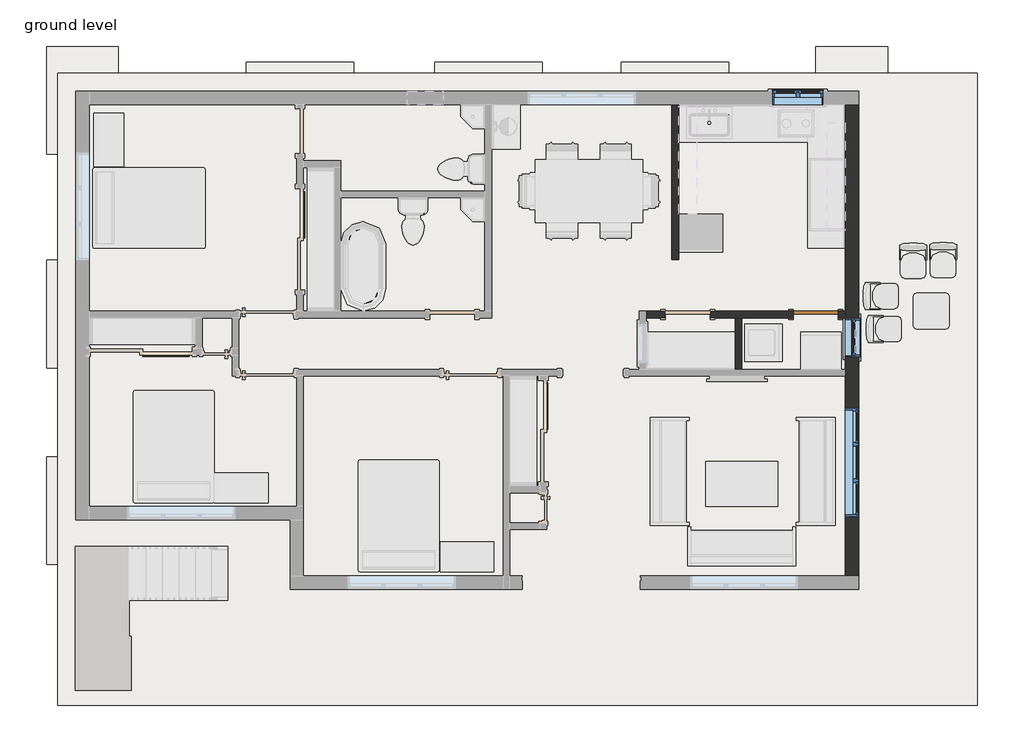
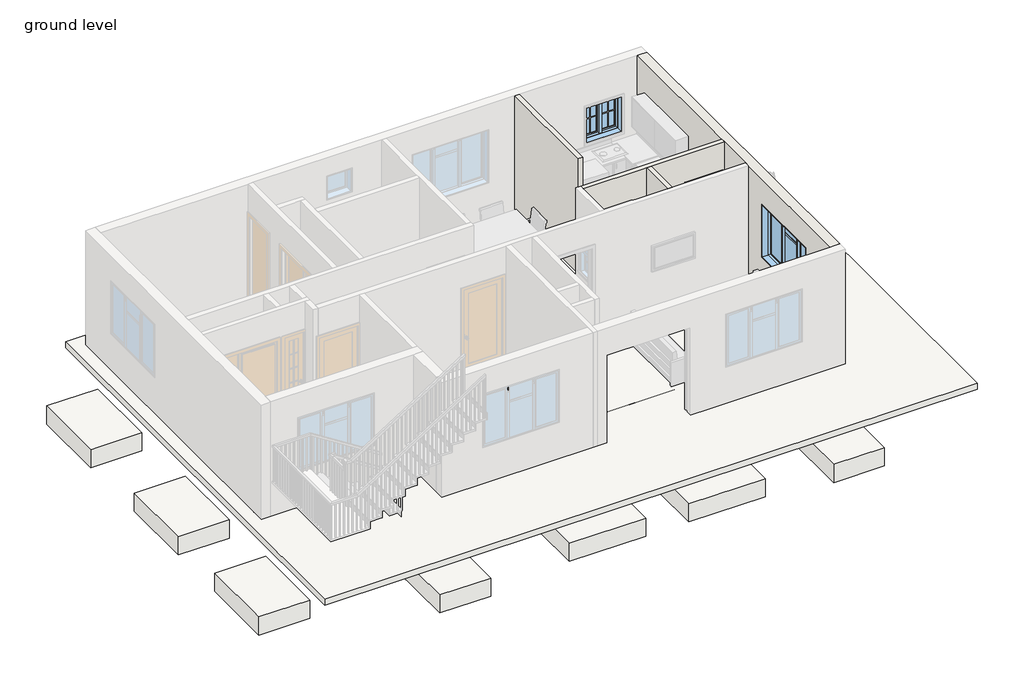
# One storey, part 2 of 4: 18 beams, 15 slabs, 4 walls, 3 windows, 1 door.
"""IFC4 building model written with IfcOpenShell, lengths in millimetres."""

from ifc_helpers import new_model, si_unit, frame, origin, place, context, project, spatial, polyline, outline, extrude, faceted_brep, transform, mapped, element, save
from components import door_214872d5, window_339605e1, window_7a1f68bc, window_251dd907

model = new_model("IFC4")

# Units and contexts
model_context = context("Model", 3, world=origin())
ifc_project = project(units=[si_unit("LENGTHUNIT", "METRE", prefix="MILLI")], contexts=[model_context])

# Site, building, storey
site = spatial("IfcSite", under=ifc_project)
building = spatial("IfcBuilding", under=site)
storey = spatial("IfcBuildingStorey", under=building, Name="ground level", Elevation=609.6)

# Beams
placement = place(None, origin())
element("IfcBeam", 1, ObjectType="Concrete-Rectangular Beam", at=placement, inside=storey, context=model_context, shape_type="Brep", body=[
    faceted_brep([(-8931.9263529, 6644.5661978, 609.6), (-8931.9263529, 6415.9661978, 609.6), (-5521.9763529, 6415.9661978, 609.6), (-5293.3763529, 6415.9661978, 609.6), (-2264.4263529, 6415.9661978, 609.6), (-2035.8263529, 6415.9661978, 609.6), (897.8736471, 6415.9661978, 609.6), (1126.4736471, 6415.9661978, 609.6), (3901.4236471, 6415.9661978, 609.6), (3901.4236471, 6644.5661978, 609.6), (1164.5736471, 6644.5661978, 609.6), (1164.5736471, 6454.0661978, 609.6), (859.7736471, 6454.0661978, 609.6), (859.7736471, 6644.5661978, 609.6), (-1997.7263529, 6644.5661978, 609.6), (-1997.7263529, 6454.0661978, 609.6), (-2302.5263529, 6454.0661978, 609.6), (-2302.5263529, 6644.5661978, 609.6), (-5198.1263529, 6644.5661978, 609.6), (-5198.1263529, 6454.0661978, 609.6), (-5502.9263529, 6454.0661978, 609.6), (-5502.9263529, 6644.5661978, 609.6), (-8931.9263529, 6415.9661978, 304.8), (-5521.9763529, 6415.9661978, 304.8), (-5293.3763529, 6415.9661978, 304.8), (-2264.4263529, 6415.9661978, 304.8), (-2035.8263529, 6415.9661978, 304.8), (897.8736471, 6415.9661978, 304.8), (1126.4736471, 6415.9661978, 304.8), (3901.4236471, 6415.9661978, 304.8), (-8931.9263529, 6644.5661978, 304.8), (-5502.9263529, 6644.5661978, 304.8), (-5502.9263529, 6454.0661978, 304.8), (-5198.1263529, 6454.0661978, 304.8), (-5198.1263529, 6644.5661978, 304.8), (-2302.5263529, 6644.5661978, 304.8), (-2302.5263529, 6454.0661978, 304.8), (-1997.7263529, 6454.0661978, 304.8), (-1997.7263529, 6644.5661978, 304.8), (859.7736471, 6644.5661978, 304.8), (859.7736471, 6454.0661978, 304.8), (1164.5736471, 6454.0661978, 304.8), (1164.5736471, 6644.5661978, 304.8), (3901.4236471, 6644.5661978, 304.8)], [[[0, 1, 2, 3, 4, 5, 6, 7, 8, 9, 10, 11, 12, 13, 14, 15, 16, 17, 18, 19, 20, 21]], [[1, 22, 23, 24, 25, 26, 27, 28, 29, 8, 7, 6, 5, 4, 3, 2]], [[22, 30, 31, 32, 33, 34, 35, 36, 37, 38, 39, 40, 41, 42, 43, 29, 28, 27, 26, 25, 24, 23]], [[42, 10, 9, 43]], [[1, 0, 30, 22]], [[33, 19, 18, 34]], [[19, 33, 32, 20]], [[20, 32, 31, 21]], [[37, 15, 14, 38]], [[15, 37, 36, 16]], [[16, 36, 35, 17]], [[41, 11, 10, 42]], [[11, 41, 40, 12]], [[12, 40, 39, 13]], [[9, 8, 29, 43]], [[30, 0, 21, 31]], [[34, 18, 17, 35]], [[38, 14, 13, 39]]]),
])
element("IfcBeam", 2, ObjectType="Concrete-Rectangular Beam", at=placement, inside=storey, context=model_context, shape_type="Brep", body=[
    faceted_brep([(4130.0236471, 1748.7161978, 609.6), (3901.4236471, 1748.7161978, 609.6), (3901.4236471, 1729.6661978, 609.6), (3901.4236471, 34.2161978, 609.6), (3901.4236471, -194.3838022, 609.6), (3901.4236471, -588.0838022, 609.6), (3901.4236471, -816.6838022, 609.6), (3901.4236471, -1470.7338022, 609.6), (4130.0236471, -1470.7338022, 609.6), (3901.4236471, 1748.7161978, 304.8), (3901.4236471, 1729.6661978, 304.8), (3901.4236471, 34.2161978, 304.8), (3901.4236471, -194.3838022, 304.8), (3901.4236471, -588.0838022, 304.8), (3901.4236471, -816.6838022, 304.8), (3901.4236471, -1470.7338022, 304.8), (4130.0236471, 1748.7161978, 304.8), (4130.0236471, -1470.7338022, 304.8)], [[[0, 1, 2, 3, 4, 5, 6, 7, 8]], [[1, 9, 10, 11, 12, 13, 14, 15, 7, 6, 5, 4, 3, 2]], [[9, 16, 17, 15, 14, 13, 12, 11, 10]], [[16, 0, 8, 17]], [[1, 0, 16, 9]], [[8, 7, 15, 17]]]),
    faceted_brep([(3901.4236471, 6377.8661978, 609.6), (4130.0236471, 6377.8661978, 609.6), (4130.0236471, 6377.8661978, 304.8), (3901.4236471, 6377.8661978, 304.8), (4130.0236471, 2053.5161978, 609.6), (3901.4236471, 2053.5161978, 609.6), (3901.4236471, 2053.5161978, 304.8), (4130.0236471, 2053.5161978, 304.8), (3901.4236471, 5558.7161978, 609.6), (3901.4236471, 5330.1161978, 609.6), (3901.4236471, 5044.3661978, 609.6), (3901.4236471, 4815.7661978, 609.6), (3901.4236471, 3012.3661978, 609.6), (3901.4236471, 2783.7661978, 609.6), (3901.4236471, 5558.7161978, 304.8), (3901.4236471, 5330.1161978, 304.8), (3901.4236471, 5044.3661978, 304.8), (3901.4236471, 4815.7661978, 304.8), (3901.4236471, 3012.3661978, 304.8), (3901.4236471, 2783.7661978, 304.8)], [[[0, 1, 2, 3]], [[4, 5, 6, 7]], [[1, 0, 8, 9, 10, 11, 12, 13, 5, 4]], [[0, 3, 14, 15, 16, 17, 18, 19, 6, 5, 13, 12, 11, 10, 9, 8]], [[3, 2, 7, 6, 19, 18, 17, 16, 15, 14]], [[2, 1, 4, 7]]]),
])
element("IfcBeam", 3, ObjectType="Concrete-Rectangular Beam", at=placement, inside=storey, context=model_context, shape_type="Brep", body=[
    faceted_brep([(3901.4236471, -1737.4338022, 609.6), (3901.4236471, -1508.8338022, 609.6), (-1731.0263529, -1508.8338022, 609.6), (-1959.6263529, -1508.8338022, 609.6), (-5293.3763529, -1508.8338022, 609.6), (-5293.3763529, -1737.4338022, 609.6), (-1997.7263529, -1737.4338022, 609.6), (-1997.7263529, -1546.9338022, 609.6), (-1692.9263529, -1546.9338022, 609.6), (-1692.9263529, -1737.4338022, 609.6), (859.7736471, -1737.4338022, 609.6), (859.7736471, -1546.9338022, 609.6), (1164.5736471, -1546.9338022, 609.6), (1164.5736471, -1737.4338022, 609.6), (3901.4236471, -1508.8338022, 304.8), (-1731.0263529, -1508.8338022, 304.8), (-1959.6263529, -1508.8338022, 304.8), (-5293.3763529, -1508.8338022, 304.8), (3901.4236471, -1737.4338022, 304.8), (1164.5736471, -1737.4338022, 304.8), (1164.5736471, -1546.9338022, 304.8), (859.7736471, -1546.9338022, 304.8), (859.7736471, -1737.4338022, 304.8), (-1692.9263529, -1737.4338022, 304.8), (-1692.9263529, -1546.9338022, 304.8), (-1997.7263529, -1546.9338022, 304.8), (-1997.7263529, -1737.4338022, 304.8), (-5293.3763529, -1737.4338022, 304.8)], [[[0, 1, 2, 3, 4, 5, 6, 7, 8, 9, 10, 11, 12, 13]], [[1, 14, 15, 16, 17, 4, 3, 2]], [[14, 18, 19, 20, 21, 22, 23, 24, 25, 26, 27, 17, 16, 15]], [[26, 6, 5, 27]], [[1, 0, 18, 14]], [[21, 11, 10, 22]], [[11, 21, 20, 12]], [[12, 20, 19, 13]], [[25, 7, 6, 26]], [[7, 25, 24, 8]], [[8, 24, 23, 9]], [[5, 4, 17, 27]], [[18, 0, 13, 19]], [[22, 10, 9, 23]]]),
])
element("IfcBeam", 4, ObjectType="Concrete-Rectangular Beam", at=placement, inside=storey, context=model_context, shape_type="Brep", body=[
    faceted_brep([(-5293.3763529, 6415.9661978, 609.6), (-5521.9763529, 6415.9661978, 609.6), (-5521.9763529, 3012.3661978, 609.6), (-5521.9763529, 2783.7661978, 609.6), (-5521.9763529, 1958.2661978, 609.6), (-5521.9763529, 1729.6661978, 609.6), (-5521.9763529, -327.7338022, 609.6), (-5521.9763529, -556.3338022, 609.6), (-5521.9763529, -1470.7338022, 609.6), (-5293.3763529, -1470.7338022, 609.6), (-5293.3763529, 1729.6661978, 609.6), (-5401.3263529, 1729.6661978, 609.6), (-5401.3263529, 1958.2661978, 609.6), (-5293.3763529, 1958.2661978, 609.6), (-5293.3763529, 2783.7661978, 609.6), (-5293.3763529, 3012.3661978, 609.6), (-5293.3763529, 5330.1161978, 609.6), (-5293.3763529, 5558.7161978, 609.6), (-5293.3763529, 6415.9661978, 304.8), (-5293.3763529, 1958.2661978, 304.8), (-5293.3763529, 2783.7661978, 304.8), (-5293.3763529, 3012.3661978, 304.8), (-5293.3763529, 5330.1161978, 304.8), (-5293.3763529, 5558.7161978, 304.8), (-5521.9763529, 6415.9661978, 304.8), (-5401.3263529, 1958.2661978, 304.8), (-5401.3263529, 1729.6661978, 304.8), (-5293.3763529, 1729.6661978, 304.8), (-5293.3763529, -1470.7338022, 304.8), (-5521.9763529, -1470.7338022, 304.8), (-5521.9763529, -556.3338022, 304.8), (-5521.9763529, -327.7338022, 304.8), (-5521.9763529, 1729.6661978, 304.8), (-5521.9763529, 1958.2661978, 304.8), (-5521.9763529, 2783.7661978, 304.8), (-5521.9763529, 3012.3661978, 304.8)], [[[0, 1, 2, 3, 4, 5, 6, 7, 8, 9, 10, 11, 12, 13, 14, 15, 16, 17]], [[18, 0, 17, 16, 15, 14, 13, 19, 20, 21, 22, 23]], [[24, 18, 23, 22, 21, 20, 19, 25, 26, 27, 28, 29, 30, 31, 32, 33, 34, 35]], [[1, 24, 35, 34, 33, 32, 31, 30, 29, 8, 7, 6, 5, 4, 3, 2]], [[1, 0, 18, 24]], [[9, 8, 29, 28]], [[12, 25, 19, 13]], [[26, 11, 10, 27]], [[11, 26, 25, 12]], [[9, 28, 27, 10]]]),
])
element("IfcBeam", 5, ObjectType="Concrete-Rectangular Beam", at=placement, inside=storey, context=model_context, shape_type="SweptSolid", body=[
    extrude(outline(polyline([(-5521.9763529, -327.7338022), (-5521.9763529, -556.3338022), (-8931.9263529, -556.3338022), (-8931.9263529, -327.7338022), (-5521.9763529, -327.7338022)])), frame((0.0, 0.0, 304.8), z_axis=(0.0, 0.0, 1.0), x_axis=(1.0, 0.0, 0.0)), (0.0, 0.0, 1.0), 304.8),
])
element("IfcBeam", 6, ObjectType="Concrete-Rectangular Beam", at=placement, inside=storey, context=model_context, shape_type="Brep", body=[
    faceted_brep([(-9160.5263529, 6720.7661978, 609.6), (-8931.9263529, 6720.7661978, 609.6), (-8931.9263529, 6720.7661978, 304.8), (-9160.5263529, 6720.7661978, 304.8), (-9160.5263529, 6682.6661978, 609.6), (-8931.9263529, 6682.6661978, 609.6), (-8931.9263529, 6682.6661978, 304.8), (-9160.5263529, 6682.6661978, 304.8)], [[[0, 1, 2, 3]], [[1, 0, 4, 5]], [[2, 1, 5, 6]], [[3, 2, 6, 7]], [[0, 3, 7, 4]], [[5, 4, 7, 6]]]),
    faceted_brep([(-9160.5263529, 6377.8661978, 609.6), (-8931.9263529, 6377.8661978, 609.6), (-8931.9263529, 6377.8661978, 304.8), (-9160.5263529, 6377.8661978, 304.8), (-8931.9263529, 3050.4661978, 609.6), (-9160.5263529, 3050.4661978, 609.6), (-9160.5263529, 3050.4661978, 304.8), (-8931.9263529, 3050.4661978, 304.8)], [[[0, 1, 2, 3]], [[4, 5, 6, 7]], [[1, 0, 5, 4]], [[2, 1, 4, 7]], [[3, 2, 7, 6]], [[0, 3, 6, 5]]]),
    faceted_brep([(-8931.9263529, -289.6338022, 609.6), (-9160.5263529, -289.6338022, 609.6), (-9160.5263529, -289.6338022, 304.8), (-8931.9263529, -289.6338022, 304.8), (-9160.5263529, 2745.6661978, 609.6), (-8931.9263529, 2745.6661978, 609.6), (-8931.9263529, 2745.6661978, 304.8), (-9160.5263529, 2745.6661978, 304.8), (-8931.9263529, 1729.6661978, 609.6), (-8931.9263529, 1958.2661978, 609.6), (-8931.9263529, 1729.6661978, 304.8), (-8931.9263529, 1958.2661978, 304.8)], [[[0, 1, 2, 3]], [[4, 5, 6, 7]], [[1, 0, 8, 9, 5, 4]], [[0, 3, 10, 11, 6, 5, 9, 8]], [[3, 2, 7, 6, 11, 10]], [[2, 1, 4, 7]]]),
])
element("IfcBeam", 7, ObjectType="Concrete-Rectangular Beam", at=placement, inside=storey, context=model_context, shape_type="Brep", body=[
    faceted_brep([(-8931.9263529, 3012.3661978, 609.6), (-8931.9263529, 2783.7661978, 609.6), (-5521.9763529, 2783.7661978, 609.6), (-5521.9763529, 3012.3661978, 609.6), (-8931.9263529, 2783.7661978, 304.8), (-5521.9763529, 2783.7661978, 304.8), (-8931.9263529, 3012.3661978, 304.8), (-5521.9763529, 3012.3661978, 304.8)], [[[0, 1, 2, 3]], [[1, 4, 5, 2]], [[4, 6, 7, 5]], [[6, 0, 3, 7]], [[1, 0, 6, 4]], [[3, 2, 5, 7]]]),
    faceted_brep([(3901.4236471, 3012.3661978, 609.6), (3901.4236471, 2783.7661978, 609.6), (3901.4236471, 2783.7661978, 304.8), (3901.4236471, 3012.3661978, 304.8), (-5293.3763529, 2783.7661978, 609.6), (-5293.3763529, 3012.3661978, 609.6), (-5293.3763529, 3012.3661978, 304.8), (-5293.3763529, 2783.7661978, 304.8), (1126.4736471, 3012.3661978, 609.6), (897.8736471, 3012.3661978, 609.6), (-2035.8263529, 3012.3661978, 609.6), (-2264.4263529, 3012.3661978, 609.6), (-4601.2263529, 3012.3661978, 609.6), (-4829.8263529, 3012.3661978, 609.6), (351.7736471, 2783.7661978, 609.6), (580.3736471, 2783.7661978, 609.6), (1977.3736471, 2783.7661978, 609.6), (2205.9736471, 2783.7661978, 609.6), (351.7736471, 2783.7661978, 304.8), (580.3736471, 2783.7661978, 304.8), (1977.3736471, 2783.7661978, 304.8), (2205.9736471, 2783.7661978, 304.8), (-4829.8263529, 3012.3661978, 304.8), (-4601.2263529, 3012.3661978, 304.8), (-2264.4263529, 3012.3661978, 304.8), (-2035.8263529, 3012.3661978, 304.8), (897.8736471, 3012.3661978, 304.8), (1126.4736471, 3012.3661978, 304.8)], [[[0, 1, 2, 3]], [[4, 5, 6, 7]], [[1, 0, 8, 9, 10, 11, 12, 13, 5, 4, 14, 15, 16, 17]], [[2, 1, 17, 16, 15, 14, 4, 7, 18, 19, 20, 21]], [[3, 2, 21, 20, 19, 18, 7, 6, 22, 23, 24, 25, 26, 27]], [[0, 3, 27, 26, 25, 24, 23, 22, 6, 5, 13, 12, 11, 10, 9, 8]]]),
])
element("IfcBeam", 8, ObjectType="Concrete-Rectangular Beam", at=placement, inside=storey, context=model_context, shape_type="Brep", body=[
    faceted_brep([(-8931.9263529, 1958.2661978, 609.6), (-8931.9263529, 1729.6661978, 609.6), (-5521.9763529, 1729.6661978, 609.6), (-5521.9763529, 1958.2661978, 609.6), (-8931.9263529, 1729.6661978, 304.8), (-5521.9763529, 1729.6661978, 304.8), (-8931.9263529, 1958.2661978, 304.8), (-5521.9763529, 1958.2661978, 304.8)], [[[0, 1, 2, 3]], [[1, 4, 5, 2]], [[4, 6, 7, 5]], [[6, 0, 3, 7]], [[1, 0, 6, 4]], [[3, 2, 5, 7]]]),
    faceted_brep([(3901.4236471, 1958.2661978, 609.6), (3901.4236471, 1748.7161978, 609.6), (3901.4236471, 1729.6661978, 609.6), (3901.4236471, 1729.6661978, 304.8), (3901.4236471, 1748.7161978, 304.8), (3901.4236471, 1958.2661978, 304.8), (618.4736471, 1729.6661978, 609.6), (618.4736471, 1958.2661978, 609.6), (618.4736471, 1958.2661978, 304.8), (618.4736471, 1729.6661978, 304.8), (2205.9736471, 1958.2661978, 609.6), (1977.3736471, 1958.2661978, 609.6), (1977.3736471, 1958.2661978, 304.8), (2205.9736471, 1958.2661978, 304.8)], [[[0, 1, 2, 3, 4, 5]], [[6, 7, 8, 9]], [[2, 1, 0, 10, 11, 7, 6]], [[3, 2, 6, 9]], [[5, 4, 3, 9, 8, 12, 13]], [[0, 5, 13, 12, 8, 7, 11, 10]]]),
    faceted_brep([(-5096.5263529, 1729.6661978, 609.6), (-5096.5263529, 1958.2661978, 609.6), (-5096.5263529, 1958.2661978, 304.8), (-5096.5263529, 1729.6661978, 304.8), (313.6736471, 1958.2661978, 609.6), (313.6736471, 1729.6661978, 609.6), (313.6736471, 1729.6661978, 304.8), (313.6736471, 1958.2661978, 304.8), (-1959.6263529, 1729.6661978, 609.6), (-1731.0263529, 1729.6661978, 609.6), (-1959.6263529, 1729.6661978, 304.8), (-1731.0263529, 1729.6661978, 304.8)], [[[0, 1, 2, 3]], [[4, 5, 6, 7]], [[1, 0, 8, 9, 5, 4]], [[0, 3, 10, 11, 6, 5, 9, 8]], [[3, 2, 7, 6, 11, 10]], [[2, 1, 4, 7]]]),
])
element("IfcBeam", 9, ObjectType="Concrete-Rectangular Beam", at=placement, inside=storey, context=model_context, shape_type="Brep", body=[
    faceted_brep([(-1959.6263529, -1508.8338022, 609.6), (-1731.0263529, -1508.8338022, 609.6), (-1731.0263529, -816.6838022, 609.6), (-1731.0263529, -588.0838022, 609.6), (-1731.0263529, -194.3838022, 609.6), (-1731.0263529, 34.2161978, 609.6), (-1731.0263529, 1729.6661978, 609.6), (-1959.6263529, 1729.6661978, 609.6), (-1959.6263529, -1508.8338022, 304.8), (-1959.6263529, 1729.6661978, 304.8), (-1731.0263529, -1508.8338022, 304.8), (-1731.0263529, 1729.6661978, 304.8), (-1731.0263529, 34.2161978, 304.8), (-1731.0263529, -194.3838022, 304.8), (-1731.0263529, -588.0838022, 304.8), (-1731.0263529, -816.6838022, 304.8)], [[[0, 1, 2, 3, 4, 5, 6, 7]], [[8, 0, 7, 9]], [[10, 8, 9, 11, 12, 13, 14, 15]], [[1, 10, 15, 14, 13, 12, 11, 6, 5, 4, 3, 2]], [[1, 0, 8, 10]], [[7, 6, 11, 9]]]),
])
element("IfcBeam", 10, ObjectType="Concrete-Rectangular Beam", at=placement, inside=storey, context=model_context, shape_type="SweptSolid", body=[
    extrude(outline(polyline([(3901.4236471, -588.0838022), (3901.4236471, -816.6838022), (-1731.0263529, -816.6838022), (-1731.0263529, -588.0838022), (3901.4236471, -588.0838022)])), frame((0.0, 0.0, 304.8), z_axis=(0.0, 0.0, 1.0), x_axis=(1.0, 0.0, 0.0)), (0.0, 0.0, 1.0), 304.8),
])
element("IfcBeam", 11, ObjectType="Concrete-Rectangular Beam", at=placement, inside=storey, context=model_context, shape_type="SweptSolid", body=[
    extrude(outline(polyline([(3901.4236471, 34.2161978), (3901.4236471, -194.3838022), (-1731.0263529, -194.3838022), (-1731.0263529, 34.2161978), (3901.4236471, 34.2161978)])), frame((0.0, 0.0, 304.8), z_axis=(0.0, 0.0, 1.0), x_axis=(1.0, 0.0, 0.0)), (0.0, 0.0, 1.0), 304.8),
])
element("IfcBeam", 12, ObjectType="Concrete-Rectangular Beam", at=placement, inside=storey, context=model_context, shape_type="Brep", body=[
    faceted_brep([(3901.4236471, 5330.1161978, 609.6), (3901.4236471, 5558.7161978, 609.6), (1126.4736471, 5558.7161978, 609.6), (897.8736471, 5558.7161978, 609.6), (-2035.8263529, 5558.7161978, 609.6), (-2264.4263529, 5558.7161978, 609.6), (-5293.3763529, 5558.7161978, 609.6), (-5293.3763529, 5330.1161978, 609.6), (-4829.8263529, 5330.1161978, 609.6), (-4601.2263529, 5330.1161978, 609.6), (-2264.4263529, 5330.1161978, 609.6), (-2035.8263529, 5330.1161978, 609.6), (897.8736471, 5330.1161978, 609.6), (1126.4736471, 5330.1161978, 609.6), (3901.4236471, 5330.1161978, 304.8), (-5293.3763529, 5330.1161978, 304.8), (-4829.8263529, 5330.1161978, 304.8), (-4601.2263529, 5330.1161978, 304.8), (-2264.4263529, 5330.1161978, 304.8), (-2035.8263529, 5330.1161978, 304.8), (897.8736471, 5330.1161978, 304.8), (1126.4736471, 5330.1161978, 304.8), (3901.4236471, 5558.7161978, 304.8), (-5293.3763529, 5558.7161978, 304.8), (-2264.4263529, 5558.7161978, 304.8), (-2035.8263529, 5558.7161978, 304.8), (897.8736471, 5558.7161978, 304.8), (1126.4736471, 5558.7161978, 304.8)], [[[0, 1, 2, 3, 4, 5, 6, 7, 8, 9, 10, 11, 12, 13]], [[14, 0, 13, 12, 11, 10, 9, 8, 7, 15, 16, 17, 18, 19, 20, 21]], [[22, 14, 21, 20, 19, 18, 17, 16, 15, 23, 24, 25, 26, 27]], [[1, 22, 27, 26, 25, 24, 23, 6, 5, 4, 3, 2]], [[1, 0, 14, 22]], [[7, 6, 23, 15]]]),
])
element("IfcBeam", 13, ObjectType="Concrete-Rectangular Beam", at=placement, inside=storey, context=model_context, shape_type="Brep", body=[
    faceted_brep([(3901.4236471, 4815.7661978, 609.6), (3901.4236471, 5044.3661978, 609.6), (1126.4736471, 5044.3661978, 609.6), (897.8736471, 5044.3661978, 609.6), (-2035.8263529, 5044.3661978, 609.6), (-2264.4263529, 5044.3661978, 609.6), (-4601.2263529, 5044.3661978, 609.6), (-4601.2263529, 4815.7661978, 609.6), (-2264.4263529, 4815.7661978, 609.6), (-2035.8263529, 4815.7661978, 609.6), (897.8736471, 4815.7661978, 609.6), (1126.4736471, 4815.7661978, 609.6), (3901.4236471, 4815.7661978, 304.8), (-4601.2263529, 4815.7661978, 304.8), (-2264.4263529, 4815.7661978, 304.8), (-2035.8263529, 4815.7661978, 304.8), (897.8736471, 4815.7661978, 304.8), (1126.4736471, 4815.7661978, 304.8), (3901.4236471, 5044.3661978, 304.8), (-4601.2263529, 5044.3661978, 304.8), (-2264.4263529, 5044.3661978, 304.8), (-2035.8263529, 5044.3661978, 304.8), (897.8736471, 5044.3661978, 304.8), (1126.4736471, 5044.3661978, 304.8)], [[[0, 1, 2, 3, 4, 5, 6, 7, 8, 9, 10, 11]], [[12, 0, 11, 10, 9, 8, 7, 13, 14, 15, 16, 17]], [[18, 12, 17, 16, 15, 14, 13, 19, 20, 21, 22, 23]], [[1, 18, 23, 22, 21, 20, 19, 6, 5, 4, 3, 2]], [[1, 0, 12, 18]], [[7, 6, 19, 13]]]),
])
element("IfcBeam", 14, ObjectType="Concrete-Rectangular Beam", at=placement, inside=storey, context=model_context, shape_type="Brep", body=[
    faceted_brep([(-4829.8263529, 3012.3661978, 609.6), (-4601.2263529, 3012.3661978, 609.6), (-4601.2263529, 4815.7661978, 609.6), (-4601.2263529, 5044.3661978, 609.6), (-4601.2263529, 5330.1161978, 609.6), (-4829.8263529, 5330.1161978, 609.6), (-4829.8263529, 3012.3661978, 304.8), (-4829.8263529, 5330.1161978, 304.8), (-4601.2263529, 3012.3661978, 304.8), (-4601.2263529, 5330.1161978, 304.8), (-4601.2263529, 5044.3661978, 304.8), (-4601.2263529, 4815.7661978, 304.8)], [[[0, 1, 2, 3, 4, 5]], [[6, 0, 5, 7]], [[8, 6, 7, 9, 10, 11]], [[1, 8, 11, 10, 9, 4, 3, 2]], [[1, 0, 6, 8]], [[5, 4, 9, 7]]]),
])
element("IfcBeam", 15, ObjectType="Concrete-Rectangular Beam", at=placement, inside=storey, context=model_context, shape_type="SweptSolid", body=[
    extrude(outline(polyline([(-2035.8263529, 3012.3661978), (-2264.4263529, 3012.3661978), (-2264.4263529, 4815.7661978), (-2035.8263529, 4815.7661978), (-2035.8263529, 3012.3661978)])), frame((0.0, 0.0, 304.8), z_axis=(0.0, 0.0, 1.0), x_axis=(1.0, 0.0, 0.0)), (0.0, 0.0, 1.0), 304.8),
    extrude(outline(polyline([(-2264.4263529, 6415.9661978), (-2035.8263529, 6415.9661978), (-2035.8263529, 5558.7161978), (-2264.4263529, 5558.7161978), (-2264.4263529, 6415.9661978)])), frame((0.0, 0.0, 304.8), z_axis=(0.0, 0.0, 1.0), x_axis=(1.0, 0.0, 0.0)), (0.0, 0.0, 1.0), 304.8),
    extrude(outline(polyline([(-2264.4263529, 5330.1161978), (-2035.8263529, 5330.1161978), (-2035.8263529, 5044.3661978), (-2264.4263529, 5044.3661978), (-2264.4263529, 5330.1161978)])), frame((0.0, 0.0, 304.8), z_axis=(0.0, 0.0, 1.0), x_axis=(1.0, 0.0, 0.0)), (0.0, 0.0, 1.0), 304.8),
])
element("IfcBeam", 16, ObjectType="Concrete-Rectangular Beam", at=placement, inside=storey, context=model_context, shape_type="SweptSolid", body=[
    extrude(outline(polyline([(1126.4736471, 3012.3661978), (897.8736471, 3012.3661978), (897.8736471, 4815.7661978), (1126.4736471, 4815.7661978), (1126.4736471, 3012.3661978)])), frame((0.0, 0.0, 304.8), z_axis=(0.0, 0.0, 1.0), x_axis=(1.0, 0.0, 0.0)), (0.0, 0.0, 1.0), 304.8),
    extrude(outline(polyline([(897.8736471, 6415.9661978), (1126.4736471, 6415.9661978), (1126.4736471, 5558.7161978), (897.8736471, 5558.7161978), (897.8736471, 6415.9661978)])), frame((0.0, 0.0, 304.8), z_axis=(0.0, 0.0, 1.0), x_axis=(1.0, 0.0, 0.0)), (0.0, 0.0, 1.0), 304.8),
    extrude(outline(polyline([(897.8736471, 5330.1161978), (1126.4736471, 5330.1161978), (1126.4736471, 5044.3661978), (897.8736471, 5044.3661978), (897.8736471, 5330.1161978)])), frame((0.0, 0.0, 304.8), z_axis=(0.0, 0.0, 1.0), x_axis=(1.0, 0.0, 0.0)), (0.0, 0.0, 1.0), 304.8),
])
element("IfcBeam", 17, ObjectType="Concrete-Rectangular Beam", at=placement, inside=storey, context=model_context, shape_type="SweptSolid", body=[
    extrude(outline(polyline([(351.7736471, 2783.7661978), (580.3736471, 2783.7661978), (580.3736471, 1958.2661978), (351.7736471, 1958.2661978), (351.7736471, 2783.7661978)])), frame((0.0, 0.0, 304.8), z_axis=(0.0, 0.0, 1.0), x_axis=(1.0, 0.0, 0.0)), (0.0, 0.0, 1.0), 304.8),
])
element("IfcBeam", 18, ObjectType="Concrete-Rectangular Beam", at=placement, inside=storey, context=model_context, shape_type="SweptSolid", body=[
    extrude(outline(polyline([(1977.3736471, 2783.7661978), (2205.9736471, 2783.7661978), (2205.9736471, 1958.2661978), (1977.3736471, 1958.2661978), (1977.3736471, 2783.7661978)])), frame((0.0, 0.0, 304.8), z_axis=(0.0, 0.0, 1.0), x_axis=(1.0, 0.0, 0.0)), (0.0, 0.0, 1.0), 304.8),
])

# Door
door_shape = door_214872d5(model_context)
element("IfcDoor", 19, ObjectType="Single-Flush : 30\" x 84\"", at=placement, inside=storey, context=model_context, shape_type="MappedRepresentation", body=[
    mapped(door_shape, transform((3406.1236471, 2891.7161978, 609.6), x_axis=(1.0, 0.0, 0.0), y_axis=(0.0, 1.0, 0.0), z_axis=(0.0, 0.0, 1.0))),
])

# Slabs
element("IfcSlab", 20, ObjectType="Footing-Rectangular : 72\" x 48\" x 18\"", at=placement, inside=storey, context=model_context, shape_type="SweptSolid", body=[
    extrude(outline(polyline([(-8436.6263529, 7444.6661978), (-8436.6263529, 5615.8661978), (-9655.8263529, 5615.8661978), (-9655.8263529, 7444.6661978), (-8436.6263529, 7444.6661978)])), frame((0.0, 0.0, -1676.4), z_axis=(0.0, 0.0, 1.0), x_axis=(1.0, 0.0, 0.0)), (0.0, 0.0, 1.0), 457.2),
])
element("IfcSlab", 21, ObjectType="Footing-Rectangular : 72\" x 48\" x 18\"", at=placement, inside=storey, context=model_context, shape_type="SweptSolid", body=[
    extrude(outline(polyline([(-6264.9263529, 7177.9661978), (-4436.1263529, 7177.9661978), (-4436.1263529, 5958.7661978), (-6264.9263529, 5958.7661978), (-6264.9263529, 7177.9661978)])), frame((0.0, 0.0, -1676.4), z_axis=(0.0, 0.0, 1.0), x_axis=(1.0, 0.0, 0.0)), (0.0, 0.0, 1.0), 457.2),
])
element("IfcSlab", 22, ObjectType="Footing-Rectangular : 72\" x 48\" x 18\"", at=placement, inside=storey, context=model_context, shape_type="SweptSolid", body=[
    extrude(outline(polyline([(-3064.5263529, 7177.9661978), (-1235.7263529, 7177.9661978), (-1235.7263529, 5958.7661978), (-3064.5263529, 5958.7661978), (-3064.5263529, 7177.9661978)])), frame((0.0, 0.0, -1676.4), z_axis=(0.0, 0.0, 1.0), x_axis=(1.0, 0.0, 0.0)), (0.0, 0.0, 1.0), 457.2),
])
element("IfcSlab", 23, ObjectType="Footing-Rectangular : 72\" x 48\" x 18\"", at=placement, inside=storey, context=model_context, shape_type="SweptSolid", body=[
    extrude(outline(polyline([(97.7736471, 7177.9661978), (1926.5736471, 7177.9661978), (1926.5736471, 5958.7661978), (97.7736471, 5958.7661978), (97.7736471, 7177.9661978)])), frame((0.0, 0.0, -1676.4), z_axis=(0.0, 0.0, 1.0), x_axis=(1.0, 0.0, 0.0)), (0.0, 0.0, 1.0), 457.2),
])
element("IfcSlab", 24, ObjectType="Footing-Rectangular : 72\" x 48\" x 18\"", at=placement, inside=storey, context=model_context, shape_type="SweptSolid", body=[
    extrude(outline(polyline([(3406.1236471, 5615.8661978), (3406.1236471, 7444.6661978), (4625.3236471, 7444.6661978), (4625.3236471, 5615.8661978), (3406.1236471, 5615.8661978)])), frame((0.0, 0.0, -1676.4), z_axis=(0.0, 0.0, 1.0), x_axis=(1.0, 0.0, 0.0)), (0.0, 0.0, 1.0), 457.2),
])
element("IfcSlab", 25, ObjectType="Footing-Rectangular : 72\" x 48\" x 18\"", at=placement, inside=storey, context=model_context, shape_type="SweptSolid", body=[
    extrude(outline(polyline([(3406.1236471, 986.7161978), (3406.1236471, 2815.5161978), (4625.3236471, 2815.5161978), (4625.3236471, 986.7161978), (3406.1236471, 986.7161978)])), frame((0.0, 0.0, -1676.4), z_axis=(0.0, 0.0, 1.0), x_axis=(1.0, 0.0, 0.0)), (0.0, 0.0, 1.0), 457.2),
])
element("IfcSlab", 26, ObjectType="Footing-Rectangular : 72\" x 48\" x 18\"", at=placement, inside=storey, context=model_context, shape_type="SweptSolid", body=[
    extrude(outline(polyline([(3406.1236471, -2537.5338022), (3406.1236471, -708.7338022), (4625.3236471, -708.7338022), (4625.3236471, -2537.5338022), (3406.1236471, -2537.5338022)])), frame((0.0, 0.0, -1676.4), z_axis=(0.0, 0.0, 1.0), x_axis=(1.0, 0.0, 0.0)), (0.0, 0.0, 1.0), 457.2),
])
element("IfcSlab", 27, ObjectType="Footing-Rectangular : 72\" x 48\" x 18\"", at=placement, inside=storey, context=model_context, shape_type="SweptSolid", body=[
    extrude(outline(polyline([(1926.5736471, -2270.8338022), (97.7736471, -2270.8338022), (97.7736471, -1051.6338022), (1926.5736471, -1051.6338022), (1926.5736471, -2270.8338022)])), frame((0.0, 0.0, -1676.4), z_axis=(0.0, 0.0, 1.0), x_axis=(1.0, 0.0, 0.0)), (0.0, 0.0, 1.0), 457.2),
])
element("IfcSlab", 28, ObjectType="Footing-Rectangular : 72\" x 48\" x 18\"", at=placement, inside=storey, context=model_context, shape_type="SweptSolid", body=[
    extrude(outline(polyline([(-930.9263529, -2270.8338022), (-2759.7263529, -2270.8338022), (-2759.7263529, -1051.6338022), (-930.9263529, -1051.6338022), (-930.9263529, -2270.8338022)])), frame((0.0, 0.0, -1676.4), z_axis=(0.0, 0.0, 1.0), x_axis=(1.0, 0.0, 0.0)), (0.0, 0.0, 1.0), 457.2),
])
element("IfcSlab", 29, ObjectType="Footing-Rectangular : 72\" x 48\" x 18\"", at=placement, inside=storey, context=model_context, shape_type="SweptSolid", body=[
    extrude(outline(polyline([(-4798.0763529, -708.7338022), (-4798.0763529, -2537.5338022), (-6017.2763529, -2537.5338022), (-6017.2763529, -708.7338022), (-4798.0763529, -708.7338022)])), frame((0.0, 0.0, -1676.4), z_axis=(0.0, 0.0, 1.0), x_axis=(1.0, 0.0, 0.0)), (0.0, 0.0, 1.0), 457.2),
])
element("IfcSlab", 30, ObjectType="Footing-Rectangular : 72\" x 48\" x 18\"", at=placement, inside=storey, context=model_context, shape_type="SweptSolid", body=[
    extrude(outline(polyline([(-8436.6263529, 472.3661978), (-8436.6263529, -1356.4338022), (-9655.8263529, -1356.4338022), (-9655.8263529, 472.3661978), (-8436.6263529, 472.3661978)])), frame((0.0, 0.0, -1676.4), z_axis=(0.0, 0.0, 1.0), x_axis=(1.0, 0.0, 0.0)), (0.0, 0.0, 1.0), 457.2),
])
element("IfcSlab", 31, ObjectType="Footing-Rectangular : 72\" x 48\" x 18\"", at=placement, inside=storey, context=model_context, shape_type="SweptSolid", body=[
    extrude(outline(polyline([(-8436.6263529, 3812.4661978), (-8436.6263529, 1983.6661978), (-9655.8263529, 1983.6661978), (-9655.8263529, 3812.4661978), (-8436.6263529, 3812.4661978)])), frame((0.0, 0.0, -1676.4), z_axis=(0.0, 0.0, 1.0), x_axis=(1.0, 0.0, 0.0)), (0.0, 0.0, 1.0), 457.2),
])
element("IfcSlab", 32, ObjectType="Footing-Rectangular : 72\" x 48\" x 18\"", at=placement, inside=storey, context=model_context, shape_type="SweptSolid", body=[
    extrude(outline(polyline([(-6163.3263529, 2453.5661978), (-4334.5263529, 2453.5661978), (-4334.5263529, 1234.3661978), (-6163.3263529, 1234.3661978), (-6163.3263529, 2453.5661978)])), frame((0.0, 0.0, -1676.4), z_axis=(0.0, 0.0, 1.0), x_axis=(1.0, 0.0, 0.0)), (0.0, 0.0, 1.0), 457.2),
])
element("IfcSlab", 33, ObjectType="Footing-Rectangular : 72\" x 48\" x 18\"", at=placement, inside=storey, context=model_context, shape_type="SweptSolid", body=[
    extrude(outline(polyline([(-448.3263529, 2453.5661978), (1380.4736471, 2453.5661978), (1380.4736471, 1234.3661978), (-448.3263529, 1234.3661978), (-448.3263529, 2453.5661978)])), frame((0.0, 0.0, -1676.4), z_axis=(0.0, 0.0, 1.0), x_axis=(1.0, 0.0, 0.0)), (0.0, 0.0, 1.0), 457.2),
])
element("IfcSlab", 34, ObjectType="Generic - 6\"", at=placement, inside=storey, context=model_context, shape_type="SweptSolid", body=[
    extrude(outline(polyline([(6149.3236471, 6987.4661978), (6149.3236471, -3750.3838022), (-9465.3263529, -3750.3838022), (-9465.3263529, 6987.4661978), (6149.3236471, 6987.4661978)])), frame((0.0, 0.0, 457.2), z_axis=(0.0, 0.0, 1.0), x_axis=(1.0, 0.0, 0.0)), (0.0, 0.0, 1.0), 152.4),
])

# Walls
element("IfcWall", 35, ObjectType="Generic - 4.5\"", at=placement, inside=storey, context=model_context, shape_type="SweptSolid", body=[
    extrude(outline(polyline([(1075.6736471, 6454.0661978), (1075.6736471, 3825.1661978), (961.3736471, 3825.1661978), (961.3736471, 6454.0661978), (1075.6736471, 6454.0661978)])), frame((0.0, 0.0, 609.6), z_axis=(0.0, 0.0, 1.0), x_axis=(1.0, 0.0, 0.0)), (0.0, 0.0, 1.0), 2895.6),
])
element("IfcWall", 36, ObjectType="Generic - 4.5\"", at=placement, inside=storey, context=model_context, shape_type="Brep", body=[
    faceted_brep([(1609.0736471, 2834.5661978, 2743.2), (1609.0736471, 2834.5661978, 609.6), (2034.5236471, 2834.5661978, 609.6), (2148.8236471, 2834.5661978, 609.6), (3025.1236471, 2834.5661978, 609.6), (3025.1236471, 2834.5661978, 2743.2), (3787.1236471, 2834.5661978, 2743.2), (3787.1236471, 2834.5661978, 609.6), (3901.4236471, 2834.5661978, 609.6), (3901.4236471, 2834.5661978, 3505.2), (2148.8236471, 2834.5661978, 3505.2), (2034.5236471, 2834.5661978, 3505.2), (523.2236471, 2834.5661978, 3505.2), (523.2236471, 2834.5661978, 609.6), (847.0736471, 2834.5661978, 609.6), (847.0736471, 2834.5661978, 2743.2), (3025.1236471, 2948.8661978, 609.6), (1609.0736471, 2948.8661978, 609.6), (1609.0736471, 2948.8661978, 2743.2), (847.0736471, 2948.8661978, 2743.2), (847.0736471, 2948.8661978, 609.6), (523.2236471, 2948.8661978, 609.6), (523.2236471, 2948.8661978, 3505.2), (3901.4236471, 2948.8661978, 3505.2), (3901.4236471, 2948.8661978, 609.6), (3787.1236471, 2948.8661978, 609.6), (3787.1236471, 2948.8661978, 2743.2), (3025.1236471, 2948.8661978, 2743.2)], [[[0, 1, 2, 3, 4, 5, 6, 7, 8, 9, 10, 11, 12, 13, 14, 15]], [[16, 17, 18, 19, 20, 21, 22, 23, 24, 25, 26, 27]], [[8, 7, 25, 24]], [[14, 13, 21, 20]], [[4, 3, 2, 1, 17, 16]], [[12, 11, 10, 9, 23, 22]], [[13, 12, 22, 21]], [[9, 8, 24, 23]], [[26, 25, 7, 6]], [[27, 26, 6, 5]], [[16, 27, 5, 4]], [[18, 17, 1, 0]], [[19, 18, 0, 15]], [[20, 19, 15, 14]]]),
])
element("IfcWall", 37, ObjectType="Generic - 4.5\"", at=placement, inside=storey, context=model_context, shape_type="SweptSolid", body=[
    extrude(outline(polyline([(2148.8236471, 2834.5661978), (2148.8236471, 1958.2661978), (2034.5236471, 1958.2661978), (2034.5236471, 2834.5661978), (2148.8236471, 2834.5661978)])), frame((0.0, 0.0, 609.6), z_axis=(0.0, 0.0, 1.0), x_axis=(1.0, 0.0, 0.0)), (0.0, 0.0, 1.0), 2895.6),
])
element("IfcWall", 38, ObjectType="Generic - 9\"", at=placement, inside=storey, context=model_context, shape_type="Brep", body=[
    faceted_brep([(4130.0236471, -1546.9338022, 609.6), (4130.0236471, 6454.0661978, 609.6), (4130.0236471, 6454.0661978, 3505.2), (4130.0236471, -1546.9338022, 3505.2), (4130.0236471, 2828.2161978, 2590.8), (4130.0236471, 2828.2161978, 1524.0), (4130.0236471, 2167.8161978, 1524.0), (4130.0236471, 2167.8161978, 2590.8), (4130.0236471, -537.2838022, 2870.2), (4130.0236471, 1291.5161978, 2870.2), (4130.0236471, 1291.5161978, 1524.0), (4130.0236471, -537.2838022, 1524.0), (3901.4236471, -1546.9338022, 609.6), (3901.4236471, -1546.9338022, 3505.2), (3901.4236471, 1843.9661978, 3505.2), (3901.4236471, 1958.2661978, 3505.2), (3901.4236471, 2834.5661978, 3505.2), (3901.4236471, 2948.8661978, 3505.2), (3901.4236471, 6454.0661978, 3505.2), (3901.4236471, 6454.0661978, 609.6), (3901.4236471, 2948.8661978, 609.6), (3901.4236471, 2834.5661978, 609.6), (3901.4236471, 1958.2661978, 609.6), (3901.4236471, 1843.9661978, 609.6), (3901.4236471, 2828.2161978, 2590.8), (3901.4236471, 2167.8161978, 2590.8), (3901.4236471, 2167.8161978, 1524.0), (3901.4236471, 2828.2161978, 1524.0), (3901.4236471, -537.2838022, 2870.2), (3901.4236471, -537.2838022, 1524.0), (3901.4236471, 1291.5161978, 1524.0), (3901.4236471, 1291.5161978, 2870.2)], [[[0, 1, 2, 3], [4, 5, 6, 7], [8, 9, 10, 11]], [[12, 13, 14, 15, 16, 17, 18, 19, 20, 21, 22, 23], [24, 25, 26, 27], [28, 29, 30, 31]], [[1, 0, 12, 23, 22, 21, 20, 19]], [[3, 2, 18, 17, 16, 15, 14, 13]], [[0, 3, 13, 12]], [[2, 1, 19, 18]], [[5, 4, 24, 27]], [[6, 5, 27, 26]], [[7, 6, 26, 25]], [[4, 7, 25, 24]], [[29, 28, 8, 11]], [[30, 29, 11, 10]], [[31, 30, 10, 9]], [[28, 31, 9, 8]]]),
])

# Windows
window_shape = window_339605e1(model_context)
element("IfcWindow", 39, ObjectType="Window-Casement-Double : 34\" x 36\"", at=placement, inside=storey, context=model_context, shape_type="MappedRepresentation", body=[
    mapped(window_shape, transform((3101.3236471, 6568.3661978, 787.4), x_axis=(1.0, 0.0, 0.0), y_axis=(0.0, 1.0, 0.0), z_axis=(0.0, 0.0, 1.0))),
])
window_2_shape = window_7a1f68bc(model_context)
element("IfcWindow", 40, ObjectType="Window-Casement-Triple-Middle-Transom : 72\" x 53\"", at=placement, inside=storey, context=model_context, shape_type="MappedRepresentation", body=[
    mapped(window_2_shape, transform((4015.7236471, 377.1161978, 609.6), x_axis=(0.0, -1.0, 0.0), y_axis=(1.0, 0.0, 0.0), z_axis=(0.0, 0.0, 1.0))),
])
window_3_shape = window_251dd907(model_context)
element("IfcWindow", 41, ObjectType="Window-Double-Hung : 26\" x 42\"", at=placement, inside=storey, context=model_context, shape_type="MappedRepresentation", body=[
    mapped(window_3_shape, transform((4015.7236471, 2498.0161978, 609.6), x_axis=(0.0, -1.0, 0.0), y_axis=(1.0, 0.0, 0.0), z_axis=(0.0, 0.0, 1.0))),
])

save(model, "model.ifc")

# Revit data of these elements
# Type "Concrete-Rectangular Beam"
#   Assembly Code = "B10"
#   Length [instance default] = 5' - 0"
#   b = 0' - 9"
#   h = 1' - 0"
#   Structural Material [instance default] = Concrete, Cast-in-Place gray
# Type "Single-Flush : 30\" x 84\""
#   Type Mark = "4"
#   Construction Type Id = "MDOOR"
#   Assembly Code = "C1020"
#   Analytic Construction = "Metal"
#   Thickness = 0' - 2"
#   Heat Transfer Coefficient (U) = 0.651978 BTU/(h·ft²·°F)
#   Height = 7' - 0"
#   Trim Projection Ext = 0' - 1"
#   Trim Projection Int = 0' - 1"
#   Trim Width = 0' - 3"
#   Width = 2' - 6"
#   Define Thermal Properties by = 1
#   Define Thermal Properties by = 1
#   Door Material = Door - Panel
#   Frame Material = Door - Frame
#   Visual Light Transmittance = 0
#   Solar Heat Gain Coefficient = 0
#   Function = (empty or 0)
#   Wall Closure = (empty or 0)
# Type "Footing-Rectangular : 72\" x 48\" x 18\""
#   Assembly Code = "A1010100"
#   Width = 4' - 0"
#   Length = 6' - 0"
#   Foundation Thickness = 1' - 6"
#   Structural Material [instance default] = Concrete, Cast-in-Place gray
# Type "Generic - 6\""
#   Assembly Code = "B1010"
#   Function = 0
#   Layers, outside or top first: 0' - 6" no material (function 1)
# Type "Generic - 4.5\""
#   Assembly Code = "B2010"
#   Layers, outside or top first: 0' - 4 1/2" no material (function 1)
# Type "Generic - 9\""
#   Assembly Code = "B2010"
#   Layers, outside or top first: 0' - 9" no material (function 1)
# Type "Window-Casement-Double : 34\" x 36\""
#   Type Mark = "14"
#   Fire Rating = "0.5h"
#   Assembly Code = "B2020100"
#   Analytic Construction = "Double glazing - domestic"
#   Frame Extension [instance default] = 0' - 0 1/4"
#   Window Inset [instance default] = 0' - 0"
#   Wall Thickness [instance default] = 0' - 6"
#   Interior Wall Closure [instance default] = 0' - 2 1/4"
#   Half Width = 1' - 5"
#   Visual Light Transmittance = 0.81
#   Thermal Resistance (R) = 1.8146 (h·ft²·°F)/BTU
#   Solar Heat Gain Coefficient = 0.76
#   Rough Width = 2' - 10 1/2"
#   Rough Height = 3' - 0 1/2"
#   Height = 3' - 0"
#   Heat Transfer Coefficient (U) = 0.5511 BTU/(h·ft²·°F)
#   Exterior Wall Closure [instance default] = 0' - 1 1/4"
#   Extension Jamb [instance default] = 0' - 2 1/4"
#   Default Sill Height = 3' - 0"
#   Width = 2' - 10"
#   Define Thermal Properties by = 0
#   Muntin Visibility = yes
#   Interior Trim Visibility [instance default] = yes
#   Exterior Trim Visibility [instance default] = yes
#   Extension Jamb Visibility [instance default] = yes
#   Interior Trim Material = Wood - Stained
#   Muntin Pattern = Muntin Pattern_2x2 : Muntin Pattern_2x2
#   Interior Trim = Trim-Window-Interior-Flat : Picture Frame
#   Interior Frame Material = Wood - Stained
#   Glass Panel Material = Glass
#   Exterior Trim Material = Clad - White
#   Exterior Trim = Trim-Window-Exterior-Flat : with Sill
#   Exterior Frame Material = Clad - White
#   Wall Closure = (empty or 0)
# Type "Window-Casement-Triple-Middle-Transom : 72\" x 53\""
#   Type Mark = "18"
#   Fire Rating = "0.5h"
#   Assembly Code = "B2020100"
#   Analytic Construction = "Double glazing - domestic"
#   Window Width = 2' - 0"
#   Window Inset [instance default] = 0' - 0 5/8"
#   Wall Thickness [instance default] = 0' - 6"
#   Visual Light Transmittance = 0.81
#   Transom Height Ratio = 0.3
#   Thermal Resistance (R) = 1.8146 (h·ft²·°F)/BTU
#   Solar Heat Gain Coefficient = 0.76
#   Rough Width = 6' - 0 1/2"
#   Rough Height = 4' - 5 1/2"
#   Heat Transfer Coefficient (U) = 0.5511 BTU/(h·ft²·°F)
#   Height = 4' - 5"
#   Transom Height = 1' - 3.9"
#   Frame Gap 3 [instance default] = 0' - 1 83/128"
#   Frame Gap 2 [instance default] = 0' - 0 5/8"
#   Frame Gap 1 = 0' - 1 51/128"
#   Default Sill Height = 3' - 0"
#   Width = 6' - 0"
#   Frame Material = Metal - Aluminum
#   Glass Panel Material = Glass
#   Wall Closure = (empty or 0)
# Type "Window-Double-Hung : 26\" x 42\""
#   Type Mark = "11"
#   Fire Rating = "0.5h"
#   Construction Type Id = "DG-DR"
#   Assembly Code = "B2020100"
#   Analytic Construction = "Double glazing - domestic"
#   Wall Thickness [instance default] = 0' - 6"
#   Window Inset [instance default] = 0' - 0"
#   Visual Light Transmittance = 0.81
#   Thermal Resistance (R) = 1.8146 (h·ft²·°F)/BTU
#   Solar Heat Gain Coefficient = 0.76
#   Muntin Width = 1' - 8"
#   Muntin Height = 1' - 5 1/8"
#   Interior Wall Closure [instance default] = 0' - 1 1/2"
#   Rough Width = 2' - 2 1/2"
#   Rough Height = 3' - 6 1/2"
#   Frame Extension [instance default] = 0' - 1 1/4"
#   Exterior Wall Closure [instance default] = 0' - 0 1/2"
#   Extension Jamb [instance default] = 0' - 1 1/2"
#   Heat Transfer Coefficient (U) = 0.5511 BTU/(h·ft²·°F)
#   Height = 3' - 6"
#   Width = 2' - 2"
#   Define Thermal Properties by = 1
#   Top Muntin Visibility = yes
#   Indicator Visibility [instance default] = yes
#   Extension Jamb Visibility [instance default] = yes
#   Interior Trim Visibility [instance default] = yes
#   Exterior Trim Visibility [instance default] = yes
#   Define Thermal Properties by = 1
#   Bottom Muntin Visibility = yes
#   Muntin Pattern = Muntin Pattern_2x2 : Muntin Pattern_2x2
#   Interior Trim Material = Wood - Stained
#   Interior Trim = Trim-Window-Interior-Flat : Picture Frame
#   Exterior Trim Material = Clad - White
#   Exterior Trim = Trim-Window-Exterior-Flat : with Sill
#   Glass Panel Material = Glass
#   Exterior Frame Material = Clad - White
#   Interior Frame Material = Wood - Stained
#   Wall Closure = (empty or 0)
# Elements 1, 2, 3, 4, 5, 6, 7, 8, 9, 10, 11, 12, 13, 14, 15, 16, 17, 18 (IfcBeam, "Concrete-Rectangular Beam")
#   Structural Material = Concrete, Cast-in-Place gray
#   Phase Created = New Construction
#   Materials on its faces: "Concrete, Cast-in-Place gray"
# Element 19 (IfcDoor, "Single-Flush : 30\" x 84\"")
#   Phase Created = New Construction
#   Materials on its faces: "Door - Frame", "Door - Panel"
# Elements 20, 21, 22, 23, 24, 25, 26, 27, 28, 29, 30, 31, 32, 33 (IfcSlab, "Footing-Rectangular : 72\" x 48\" x 18\"")
#   Structural Material = Concrete, Cast-in-Place gray
#   Phase Created = New Construction
#   Materials on its faces: "Concrete, Cast-in-Place gray"
# Element 34 (IfcSlab, "Generic - 6\"")
#   Height Offset From Level = 0' - 0"
#   Phase Created = New Construction
#   Materials on its faces: "Default Floor"
# Elements 35, 36, 37 (IfcWall, "Generic - 4.5\"")
#   Top Offset = 0' - 0"
#   Base Offset = 0' - 0"
#   Unconnected Height = 9' - 6"
#   wall height = 9' - 6"
#   Phase Created = New Construction
#   Base Constraint = ground level
#   Materials on its faces: "Default Wall"
# Element 38 (IfcWall, "Generic - 9\"")
#   Top Offset = 0' - 0"
#   Base Offset = 0' - 0"
#   Unconnected Height = 9' - 6"
#   wall height = 9' - 6"
#   Phase Created = New Construction
#   Base Constraint = ground level
#   Materials on its faces: "Default Wall"
# Element 39 (IfcWindow, "Window-Casement-Double : 34\" x 36\"")
#   Mark = "2"
#   Window Inset = 0' - 0"
#   Interior Wall Closure = 0' - 2 1/4"
#   Frame Extension = 0' - 0 1/4"
#   Exterior Wall Closure = 0' - 1 1/4"
#   Interior Trim Visibility = yes
#   Exterior Trim Visibility = yes
#   Phase Created = New Construction
#   Materials on its faces: "Wood - Stained", "Glass", "Clad - White"
# Element 40 (IfcWindow, "Window-Casement-Triple-Middle-Transom : 72\" x 53\"")
#   Mark = "9"
#   Window Inset = 0' - 0 5/8"
#   Frame Gap 3 = 0' - 1 83/128"
#   Frame Gap 2 = 0' - 0 5/8"
#   Phase Created = New Construction
#   Materials on its faces: "Metal - Aluminum", "Glass"
# Element 41 (IfcWindow, "Window-Double-Hung : 26\" x 42\"")
#   Mark = "3"
#   Window Inset = 0' - 0"
#   Interior Wall Closure = 0' - 1 1/2"
#   Frame Extension = 0' - 1 1/4"
#   Exterior Wall Closure = 0' - 0 1/2"
#   Interior Trim Visibility = yes
#   Indicator Visibility = yes
#   Exterior Trim Visibility = yes
#   Phase Created = New Construction
#   Materials on its faces: "Wood - Stained", "Glass", "Clad - White"
# Materials
#   "Concrete, Cast-in-Place gray": class "Concrete", colour RGB 192 192 192, transparency 0, Description = "Cast-in-place concrete", Cost = 0
#   "Door - Panel": class "Wood", colour RGB 210 159 95, transparency 0, Cost = 0
#   "Door - Frame": colour RGB 118 70 51, transparency 0, Cost = 0
#   "Wood - Stained": class "Wood", colour RGB 224 178 126, transparency 0, Cost = 0
#   "Glass": class "Glass", colour RGB 0 128 192, transparency 0.75, Description = "Soda Lime Glass", Cost = 0
#   "Clad - White": class "Wood", colour RGB 242 242 238, transparency 0, Cost = 0
#   "Metal - Aluminum": class "Metal", colour RGB 247 247 247, transparency 0
#   "Default Floor": colour RGB 128 128 128, transparency 0, Cost = 0
#   "Default Wall": colour RGB 128 128 128, transparency 0, Cost = 0
